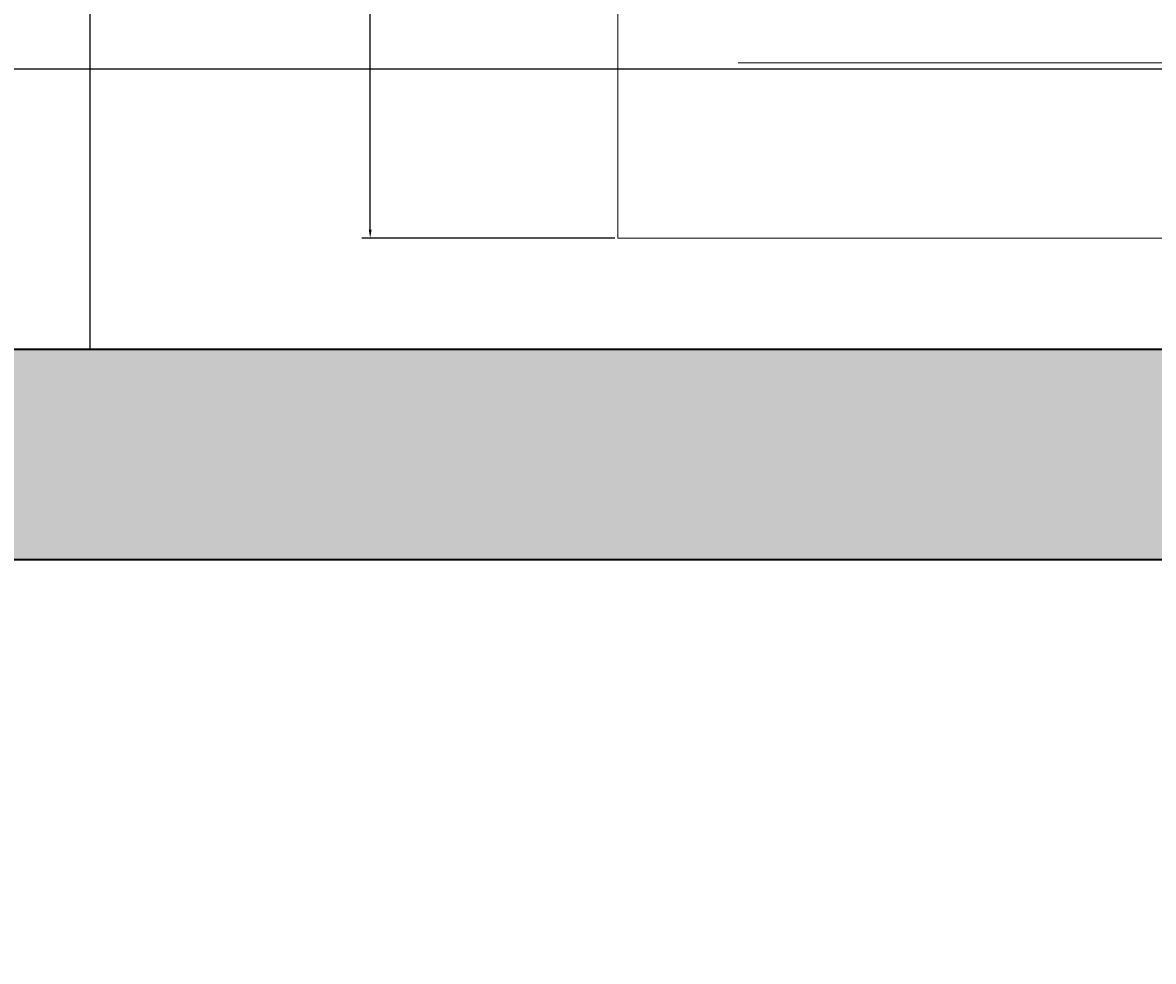
# Model space of a CAD drawing. Units: inches. Extents: x 1998 to 2588, y 1139 to 1977.
# Tile 15 of 134: x 2147 to 2171, y 1576 to 1596. Entities that reach past the tile are written whole.
import ezdxf

# ---------------------------------------------------------------- set-up
doc = ezdxf.new("R2010")
doc.units = ezdxf.units.IN
for name, color, linetype, lineweight in [('A-ANNO-DIMS', 2, 'Continuous', 18), ('A-FLOR-CASE', 32, 'Continuous', 25), ('A-FLOR-FIXT', 9, 'Continuous', 18), ('A-WALL-PATT', 252, 'Continuous', 13), ('WALL', 200, 'Continuous', 35)]:
    doc.layers.add(name, color=color, linetype=linetype, lineweight=lineweight)
doc.styles.get("Standard").update_dxf_attribs({"font": 'arial.ttf'})
doc.dimstyles.get("Standard").update_dxf_attribs({"dimtxt": 0.18, "dimasz": 0.18, "dimexe": 0.18, "dimexo": 0.0625, "dimgap": 0.09, "dimtad": 0, "dimtih": 1, "dimtoh": 1, "dimdec": 4, "dimzin": 0, "dimdsep": 46, "dimtxsty": 'Standard', "dimcen": 0.09, "dimadec": 0, "dimazin": 0, "dimtfac": 1, "dimtdec": 4, "dimtofl": 0, "dimtmove": 0, "dimatfit": 3, "dimfxl": 1, "dimtolj": 1, "dimtzin": 0, "dimarcsym": 0})

# ---------------------------------------------------------------- blocks, each defined once
blk = doc.blocks.new('SINK-WITH-DRAINBOARD')
for p, q in [((17.653, 0), (17.653, 19.174)), ((15.925, 17.391), (2.574, 17.391)), ((15.925, 15.023), (2.574, 15.023)), ((15.925, 12.848), (2.574, 12.848)), ((15.925, 10.383), (2.574, 10.383)), ((15.925, 8.143), (2.574, 8.143)), ((15.925, 5.899), (2.574, 5.899)), ((15.925, 3.752), (2.574, 3.752))]:
    blk.add_line(p, q)
blk.add_lwpolyline([(35.306, 19.174), (0, 19.174), (0, 0), (35.306, 0)], close=True)
blk.add_circle((25.956, 9.71), 1.353)
blk = doc.blocks.new('*D20')
at = {"layer": 'A-ANNO-DIMS', "color": 0, "lineweight": -2, "transparency": 16777216}
for p, q in [((2159.674, 1610.293), (2154.261, 1610.293)), ((2154.441, 1610.113), (2154.441, 1600.888)), ((2154.441, 1591.299), (2154.441, 1600.524)), ((2159.674, 1591.119), (2154.261, 1591.119))]:
    blk.add_line(p, q, dxfattribs=at)
at = {"layer": 'A-ANNO-DIMS', "color": 0, "transparency": 16777216}
for points in [[(2154.411, 1610.113), (2154.471, 1610.113), (2154.441, 1610.293)], [(2154.411, 1591.299), (2154.471, 1591.299), (2154.441, 1591.119)]]:
    blk.add_solid(points, dxfattribs=at)
at = {"layer": 'Defpoints', "color": 0, "transparency": 16777216}
for p in [(2154.441, 1610.293), (2159.737, 1610.293), (2159.737, 1591.119)]:
    blk.add_point(p, dxfattribs=at)
at = {"layer": 'A-ANNO-DIMS', "color": 0, "transparency": 16777216, "insert": (2154.441, 1600.706), "char_height": 0.18, "attachment_point": 5}
blk.add_mtext('\\A1;19 TYP.', dxfattribs=at)
blk = doc.blocks.new('*D30')
at = {"layer": 'A-ANNO-DIMS', "color": 0, "lineweight": -2, "transparency": 16777216}
for p, q in [((2407.91, 1636.732), (1997.843, 1636.732)), ((1998.023, 1636.552), (1998.023, 1615.913)), ((1998.023, 1594.912), (1998.023, 1615.552)), ((2407.91, 1594.732), (1997.843, 1594.732))]:
    blk.add_line(p, q, dxfattribs=at)
at = {"layer": 'A-ANNO-DIMS', "color": 0, "transparency": 16777216}
for points in [[(1997.993, 1636.552), (1998.053, 1636.552), (1998.023, 1636.732)], [(1997.993, 1594.912), (1998.053, 1594.912), (1998.023, 1594.732)]]:
    blk.add_solid(points, dxfattribs=at)
at = {"layer": 'Defpoints', "color": 0, "transparency": 16777216}
for p in [(1998.023, 1636.732), (2407.973, 1636.732), (2407.973, 1594.732)]:
    blk.add_point(p, dxfattribs=at)
at = {"layer": 'A-ANNO-DIMS', "color": 0, "transparency": 16777216, "insert": (1998.023, 1615.732), "char_height": 0.18, "attachment_point": 5}
blk.add_mtext('\\A1;42', dxfattribs=at)
blk = doc.blocks.new('*D34')
at = {"layer": 'A-ANNO-DIMS', "color": 0, "lineweight": -2, "transparency": 16777216}
for p, q in [((2407.91, 1594.732), (1997.843, 1594.732)), ((1998.023, 1594.552), (1998.023, 1558.913)), ((1998.023, 1522.912), (1998.023, 1558.552)), ((2407.91, 1522.732), (1997.843, 1522.732))]:
    blk.add_line(p, q, dxfattribs=at)
at = {"layer": 'A-ANNO-DIMS', "color": 0, "transparency": 16777216}
for points in [[(1997.993, 1594.552), (1998.053, 1594.552), (1998.023, 1594.732)], [(1997.993, 1522.912), (1998.053, 1522.912), (1998.023, 1522.732)]]:
    blk.add_solid(points, dxfattribs=at)
at = {"layer": 'Defpoints', "color": 0, "transparency": 16777216}
for p in [(1998.023, 1594.732), (2407.973, 1594.732), (2407.973, 1522.732)]:
    blk.add_point(p, dxfattribs=at)
at = {"layer": 'A-ANNO-DIMS', "color": 0, "transparency": 16777216, "insert": (1998.023, 1558.732), "char_height": 0.18, "attachment_point": 5}
blk.add_mtext('\\A1;72', dxfattribs=at)
blk = doc.blocks.new('*D35')
at = {"layer": 'A-ANNO-DIMS', "color": 0, "lineweight": -2, "transparency": 16777216}
for p, q in [((2148.392, 1612.732), (1997.843, 1612.732)), ((1998.023, 1612.552), (1998.023, 1600.913)), ((1998.023, 1588.912), (1998.023, 1600.552)), ((2148.392, 1588.732), (1997.843, 1588.732))]:
    blk.add_line(p, q, dxfattribs=at)
at = {"layer": 'A-ANNO-DIMS', "color": 0, "transparency": 16777216}
for points in [[(1997.993, 1612.552), (1998.053, 1612.552), (1998.023, 1612.732)], [(1997.993, 1588.912), (1998.053, 1588.912), (1998.023, 1588.732)]]:
    blk.add_solid(points, dxfattribs=at)
at = {"layer": 'Defpoints', "color": 0, "transparency": 16777216}
for p in [(1998.023, 1612.732), (2148.455, 1612.732), (2148.455, 1588.732)]:
    blk.add_point(p, dxfattribs=at)
at = {"layer": 'A-ANNO-DIMS', "color": 0, "transparency": 16777216, "insert": (1998.023, 1600.732), "char_height": 0.18, "attachment_point": 5}
blk.add_mtext('\\A1;24', dxfattribs=at)

msp = doc.modelspace()

# ---------------------------------------------------------------- hatches: boundary and pattern name
at = {"layer": 'A-WALL-PATT'}
h = msp.add_hatch(color=256, dxfattribs=at)
h.dxf.hatch_style = 1
h.paths.add_polyline_path([(2222.9729, 1888.7324), (2099.4125, 1888.7324), (2099.4125, 1879.7324), (2222.9729, 1879.7324)])
h.paths.add_polyline_path([(2096.9729, 1868.3278), (2087.9729, 1868.3278), (2087.9729, 1775.637), (2096.9729, 1775.637)])
h.paths.add_polyline_path([(2227.4729, 1868.3278), (2222.9729, 1868.3278), (2222.9729, 1774.3318), (2227.4729, 1774.3318)])
h.paths.add_polyline_path([(2188.3019, 1759.7324), (2138.6074, 1759.7324), (2099.4125, 1759.7324), (2099.4125, 1755.2324), (2176.9729, 1755.2324), (2188.3019, 1755.2324)])
h.paths.add_polyline_path([(2087.9729, 1759.7324), (2059.4729, 1759.7324), (2059.4729, 1702.7324), (2087.9729, 1702.7324), (2087.9729, 1707.2324), (2063.9729, 1707.2324), (2063.9729, 1755.2324), (2087.9729, 1755.2324)])
h.paths.add_polyline_path([(2096.9729, 1755.2324), (2087.9729, 1755.2324), (2087.9729, 1707.2324), (2096.9729, 1707.2324)])
h.paths.add_polyline_path([(2187.0461, 1707.2324), (2105.9729, 1707.2324), (2096.9729, 1707.2324), (2087.9729, 1707.2324), (2087.9729, 1702.7324), (2105.9729, 1702.7324), (2114.9729, 1702.7324), (2187.0461, 1702.7324)])
h.paths.add_polyline_path([(2181.4729, 1719.2028), (2176.9729, 1719.2028), (2176.9729, 1707.2324), (2181.4729, 1707.2324)])
h.paths.add_polyline_path([(2216.0332, 1588.7324), (2114.9729, 1588.7324), (2105.9729, 1588.7324), (2105.9729, 1584.2324), (2216.0332, 1584.2324)])
h.paths.add_polyline_path([(2077.691, 1588.7324), (2061.4729, 1588.7324), (2061.4729, 1584.2324), (2077.691, 1584.2324)])
h.paths.add_polyline_path([(2105.9729, 1588.7324), (2098.0956, 1588.7324), (2098.0956, 1584.2324), (2105.9729, 1584.2324)])
h.paths.add_polyline_path([(2114.9729, 1596.2642), (2110.1012, 1596.2642), (2105.9729, 1596.2642), (2105.9729, 1588.7324), (2114.9729, 1588.7324)])
h.paths.add_polyline_path([(2114.9729, 1584.2324), (2105.9729, 1584.2324), (2105.9729, 1580.249), (2110.1012, 1580.249), (2114.9729, 1580.249)])
h.paths.add_polyline_path([(2114.9729, 1547.7716), (2110.1012, 1547.7716, -0.0318759), (2105.9729, 1548.035), (2105.9729, 1470.2324), (2108.3775, 1470.2324), (2108.3775, 1465.7324), (2186.2943, 1465.7324), (2186.2943, 1470.2324), (2114.9729, 1470.2324)])
h.paths.add_polyline_path([(2227.4729, 1584.2324), (2222.9729, 1584.2324), (2222.9729, 1486.137), (2227.4729, 1486.137)])
h.paths.add_polyline_path([(2295.4138, 1593.2324), (2227.4729, 1593.2324), (2227.4729, 1588.7324), (2295.4138, 1588.7324), (2295.4138, 1591.8729)])
h.paths.add_polyline_path([(2345.9729, 1627.1165), (2341.4729, 1627.1165), (2341.4729, 1593.2324), (2337.2869, 1593.2324), (2337.2869, 1591.8729), (2337.2869, 1588.7324), (2345.9729, 1588.7324)])
h.paths.add_polyline_path([(2291.9729, 1588.7324), (2287.4729, 1588.7324), (2287.4729, 1522.7324), (2291.9729, 1522.7324)])
h.paths.add_polyline_path([(2291.9729, 1522.7324), (2287.4729, 1522.7324), (2227.4729, 1522.7324), (2227.4729, 1518.2324), (2291.9729, 1518.2324)])
h.paths.add_polyline_path([(2295.7347, 1519.5919), (2295.7347, 1522.7324), (2291.9729, 1522.7324), (2291.9729, 1518.2324), (2295.7347, 1518.2324)])
h.paths.add_polyline_path([(2345.9729, 1522.7324), (2337.6078, 1522.7324), (2337.6078, 1519.5919), (2337.6078, 1518.2324), (2341.4729, 1518.2324), (2341.4729, 1488.5616), (2345.9729, 1488.5616)])
h.paths.add_polyline_path([(2345.9729, 1468.1569), (2341.4729, 1468.1569), (2341.4729, 1374.2324), (2227.4729, 1374.2324), (2227.4729, 1369.7324), (2345.9729, 1369.7324)])
h.paths.add_polyline_path([(2345.9729, 1369.7324), (2341.4729, 1369.7324), (2341.4729, 1362.2324), (2345.9729, 1362.2324)])
h.paths.add_polyline_path([(2345.9729, 1317.7324), (2345.9729, 1322.2324), (2341.4729, 1322.2324), (2341.4729, 1285.137), (2345.9729, 1285.137)], flags=17)
h.paths.add_polyline_path([(2356.2096, 1322.2324), (2345.9729, 1322.2324), (2345.9729, 1317.7324), (2356.2096, 1317.7324), (2356.2096, 1319.3088)], flags=17)
h.paths.add_polyline_path([(2393.9729, 1322.2324), (2375.6999, 1322.2324), (2375.6999, 1319.3088, -0.0202458), (2375.636, 1317.7324), (2393.9729, 1317.7324)], flags=17)
h.paths.add_polyline_path([(2398.4729, 1322.2324), (2393.9729, 1322.2324), (2393.9729, 1317.7324), (2393.9729, 1237.7324), (2345.9729, 1237.7324), (2345.9729, 1264.7324), (2341.4729, 1264.7324), (2341.4729, 1228.7324), (2393.9729, 1228.7324), (2482.7412, 1228.7324), (2482.7412, 1237.7324), (2398.4729, 1237.7324), (2398.4729, 1297.1029)])
h.paths.add_polyline_path([(2398.4729, 1362.2324), (2393.9729, 1362.2324), (2393.9729, 1357.7324), (2398.4729, 1357.7324)])
h.paths.add_polyline_path([(2345.9729, 1329.7549), (2341.4729, 1329.7549), (2341.4729, 1322.2324), (2345.9729, 1322.2324)])

# ---------------------------------------------------------------- linework, layer by layer
at = {"layer": 'A-FLOR-CASE'}
msp.add_line((2148.4548, 1588.7324), (2148.4548, 1612.7324), dxfattribs=at)
at = {"layer": 'WALL'}
for p, q in [((2216.0332, 1588.7324), (2114.9729, 1588.7324)), ((2227.4729, 1584.2324), (2105.9729, 1584.2324))]:
    msp.add_line(p, q, dxfattribs=at)

# ---------------------------------------------------------------- block references
at = {"layer": 'A-FLOR-FIXT'}
msp.add_blockref('SINK-WITH-DRAINBOARD', (2159.737, 1591.119), dxfattribs=at)

# ---------------------------------------------------------------- dimensions: what is measured, and where the dimension line sits
at = {"layer": 'A-ANNO-DIMS'}
for base, p1, p2, picture, middle in [((1998.0229, 1636.7324), (2407.9729, 1594.7324), (2407.9729, 1636.7324), '*D30', (1998.0229, 1615.7324)), ((1998.0229, 1612.7324), (2148.4548, 1588.7324), (2148.4548, 1612.7324), '*D35', (1998.0229, 1600.7324)), ((1998.0229, 1594.7324), (2407.9729, 1522.7324), (2407.9729, 1594.7324), '*D34', (1998.0229, 1558.7324))]:
    dim = msp.add_linear_dim(base=base, p1=p1, p2=p2, angle=90, dimstyle='Standard', override={"dimdec": 0, "dimlfac": 1, "dimrnd": 0, "dimzin": 0, "dimdsep": 46, "dimlunit": 2}, dxfattribs=at)
    dim.commit()
    dim.dimension.update_dxf_attribs({"geometry": picture, "text_midpoint": middle})
dim = msp.add_linear_dim(base=(2154.4407, 1610.2935), p1=(2159.7366, 1591.1193), p2=(2159.7366, 1610.2935), angle=90, text='<> TYP.', dimstyle='Standard', override={"dimdec": 0, "dimlfac": 1, "dimrnd": 0, "dimzin": 0, "dimdsep": 46, "dimlunit": 2}, dxfattribs=at)
dim.commit()
dim.dimension.update_dxf_attribs({"geometry": '*D20', "text_midpoint": (2154.4407, 1600.7064)})

doc.saveas('drawing.dxf')
